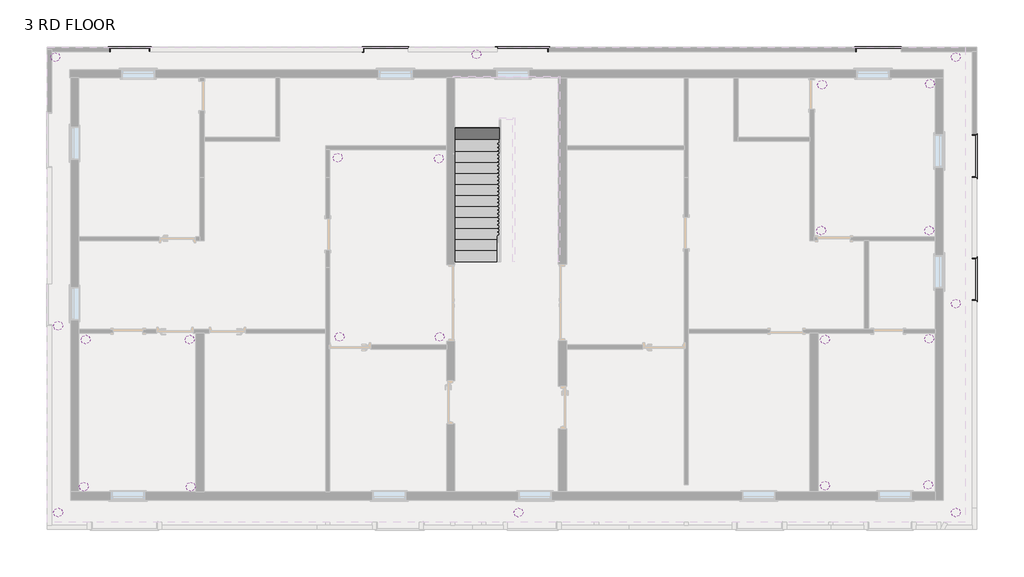
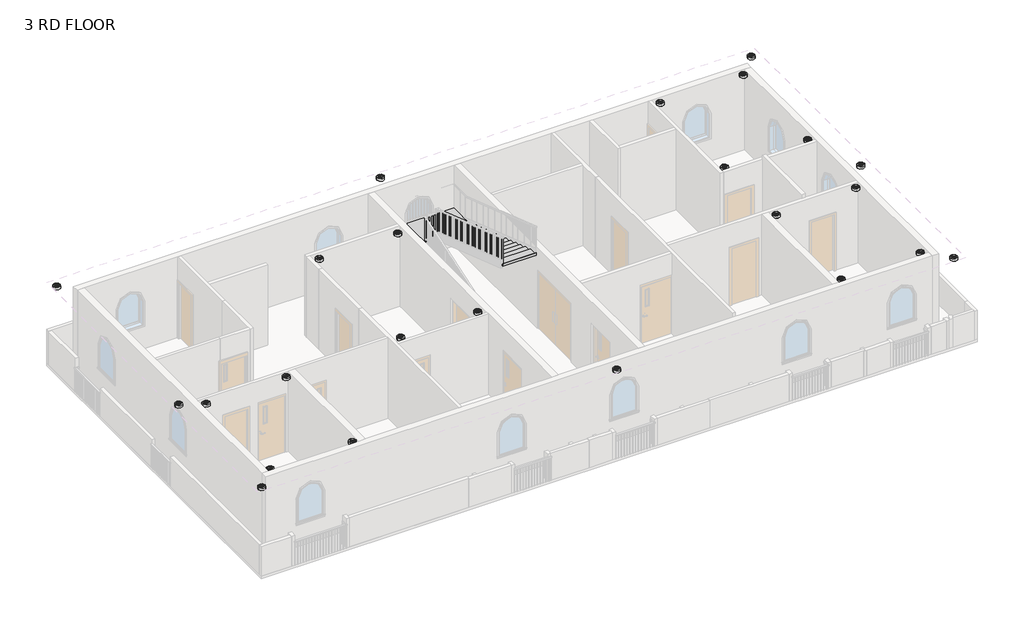
# One storey, part 6 of 7: 24 light fixtures, 6 railings, 1 stair flight.
"""IFC4 building model written with IfcOpenShell, lengths in millimetres."""

from ifc_helpers import new_model, si_unit, frame, origin, place, context, project, spatial, polyline, outline, extrude, faceted_brep, transform, mapped, element, save
from components import ceiling_light_flat_round_60w_120v_7c4c2a52, stair_flight_f733c31e

model = new_model("IFC4")

# Units and contexts
model_context = context("Model", 3, world=origin())
ifc_project = project(units=[si_unit("LENGTHUNIT", "METRE", prefix="MILLI")], contexts=[model_context])

# Site, building, storey
site = spatial("IfcSite", under=ifc_project)
building = spatial("IfcBuilding", under=site)
storey = spatial("IfcBuildingStorey", under=building, Name="3 RD FLOOR", Elevation=9601.2)

# Light fixtures
placement = place(None, origin())
ceiling_light_flat_round_60w_120v_shape = ceiling_light_flat_round_60w_120v_7c4c2a52(model_context)
element("IfcLightFixture", 1, ObjectType="Ceiling Light - Flat Round : 60W - 120V", at=placement, inside=storey, context=model_context, shape_type="MappedRepresentation", body=[
    mapped(ceiling_light_flat_round_60w_120v_shape, transform((-12872.3987925, 8203.3067329, 10210.8), x_axis=(1.0, 0.0, 0.0), y_axis=(0.0, 1.0, 0.0), z_axis=(0.0, 0.0, 1.0))),
])
element("IfcLightFixture", 2, ObjectType="Ceiling Light - Flat Round : 60W - 120V", at=placement, inside=storey, context=model_context, shape_type="MappedRepresentation", body=[
    mapped(ceiling_light_flat_round_60w_120v_shape, transform((-1251.8987998, 8279.5067329, 10210.8), x_axis=(1.0, 0.0, 0.0), y_axis=(0.0, 1.0, 0.0), z_axis=(0.0, 0.0, 1.0))),
])
element("IfcLightFixture", 3, ObjectType="Ceiling Light - Flat Round : 60W - 120V", at=placement, inside=storey, context=model_context, shape_type="MappedRepresentation", body=[
    mapped(ceiling_light_flat_round_60w_120v_shape, transform((11968.8012075, 8203.3067329, 10210.8), x_axis=(1.0, 0.0, 0.0), y_axis=(0.0, 1.0, 0.0), z_axis=(0.0, 0.0, 1.0))),
])
element("IfcLightFixture", 4, ObjectType="Ceiling Light - Flat Round : 60W - 120V", at=placement, inside=storey, context=model_context, shape_type="MappedRepresentation", body=[
    mapped(ceiling_light_flat_round_60w_120v_shape, transform((-12796.1987925, -4356.9932193, 10210.8), x_axis=(1.0, 0.0, 0.0), y_axis=(0.0, 1.0, 0.0), z_axis=(0.0, 0.0, 1.0))),
])
element("IfcLightFixture", 5, ObjectType="Ceiling Light - Flat Round : 60W - 120V", at=placement, inside=storey, context=model_context, shape_type="MappedRepresentation", body=[
    mapped(ceiling_light_flat_round_60w_120v_shape, transform((-96.7067989, -4356.9932193, 10210.8), x_axis=(1.0, 0.0, 0.0), y_axis=(0.0, 1.0, 0.0), z_axis=(0.0, 0.0, 1.0))),
])
element("IfcLightFixture", 6, ObjectType="Ceiling Light - Flat Round : 60W - 120V", at=placement, inside=storey, context=model_context, shape_type="MappedRepresentation", body=[
    mapped(ceiling_light_flat_round_60w_120v_shape, transform((11968.8012075, -4356.9932193, 10210.8), x_axis=(1.0, 0.0, 0.0), y_axis=(0.0, 1.0, 0.0), z_axis=(0.0, 0.0, 1.0))),
])
element("IfcLightFixture", 7, ObjectType="Ceiling Light - Flat Round : 60W - 120V", at=placement, inside=storey, context=model_context, shape_type="MappedRepresentation", body=[
    mapped(ceiling_light_flat_round_60w_120v_shape, transform((11968.8012075, 1402.4567334, 10210.8), x_axis=(1.0, 0.0, 0.0), y_axis=(0.0, 1.0, 0.0), z_axis=(0.0, 0.0, 1.0))),
])
element("IfcLightFixture", 8, ObjectType="Ceiling Light - Flat Round : 60W - 120V", at=placement, inside=storey, context=model_context, shape_type="MappedRepresentation", body=[
    mapped(ceiling_light_flat_round_60w_120v_shape, transform((-12796.1987925, 792.8567334, 10210.8), x_axis=(1.0, 0.0, 0.0), y_axis=(0.0, 1.0, 0.0), z_axis=(0.0, 0.0, 1.0))),
])
element("IfcLightFixture", 9, ObjectType="Ceiling Light - Flat Round : 60W - 120V", at=placement, inside=storey, context=model_context, shape_type="MappedRepresentation", body=[
    mapped(ceiling_light_flat_round_60w_120v_shape, transform((8279.4512079, 7441.3067329, 10210.8), x_axis=(1.0, 0.0, 0.0), y_axis=(0.0, 1.0, 0.0), z_axis=(0.0, 0.0, 1.0))),
])
element("IfcLightFixture", 10, ObjectType="Ceiling Light - Flat Round : 60W - 120V", at=placement, inside=storey, context=model_context, shape_type="MappedRepresentation", body=[
    mapped(ceiling_light_flat_round_60w_120v_shape, transform((11257.6012075, 7466.7067329, 10210.8), x_axis=(1.0, 0.0, 0.0), y_axis=(0.0, 1.0, 0.0), z_axis=(0.0, 0.0, 1.0))),
])
element("IfcLightFixture", 11, ObjectType="Ceiling Light - Flat Round : 60W - 120V", at=placement, inside=storey, context=model_context, shape_type="MappedRepresentation", body=[
    mapped(ceiling_light_flat_round_60w_120v_shape, transform((8254.0512079, 3421.7567332, 10210.8), x_axis=(1.0, 0.0, 0.0), y_axis=(0.0, 1.0, 0.0), z_axis=(0.0, 0.0, 1.0))),
])
element("IfcLightFixture", 12, ObjectType="Ceiling Light - Flat Round : 60W - 120V", at=placement, inside=storey, context=model_context, shape_type="MappedRepresentation", body=[
    mapped(ceiling_light_flat_round_60w_120v_shape, transform((11232.2012075, 3421.7567332, 10210.8), x_axis=(1.0, 0.0, 0.0), y_axis=(0.0, 1.0, 0.0), z_axis=(0.0, 0.0, 1.0))),
])
element("IfcLightFixture", 13, ObjectType="Ceiling Light - Flat Round : 60W - 120V", at=placement, inside=storey, context=model_context, shape_type="MappedRepresentation", body=[
    mapped(ceiling_light_flat_round_60w_120v_shape, transform((8362.0012079, 411.8567334, 10210.8), x_axis=(1.0, 0.0, 0.0), y_axis=(0.0, 1.0, 0.0), z_axis=(0.0, 0.0, 1.0))),
])
element("IfcLightFixture", 14, ObjectType="Ceiling Light - Flat Round : 60W - 120V", at=placement, inside=storey, context=model_context, shape_type="MappedRepresentation", body=[
    mapped(ceiling_light_flat_round_60w_120v_shape, transform((11232.2012075, 437.2567334, 10210.8), x_axis=(1.0, 0.0, 0.0), y_axis=(0.0, 1.0, 0.0), z_axis=(0.0, 0.0, 1.0))),
])
element("IfcLightFixture", 15, ObjectType="Ceiling Light - Flat Round : 60W - 120V", at=placement, inside=storey, context=model_context, shape_type="MappedRepresentation", body=[
    mapped(ceiling_light_flat_round_60w_120v_shape, transform((8362.0012079, -3620.3932193, 10210.8), x_axis=(1.0, 0.0, 0.0), y_axis=(0.0, 1.0, 0.0), z_axis=(0.0, 0.0, 1.0))),
])
element("IfcLightFixture", 16, ObjectType="Ceiling Light - Flat Round : 60W - 120V", at=placement, inside=storey, context=model_context, shape_type="MappedRepresentation", body=[
    mapped(ceiling_light_flat_round_60w_120v_shape, transform((11206.8012075, -3594.9932193, 10210.8), x_axis=(1.0, 0.0, 0.0), y_axis=(0.0, 1.0, 0.0), z_axis=(0.0, 0.0, 1.0))),
])
element("IfcLightFixture", 17, ObjectType="Ceiling Light - Flat Round : 60W - 120V", at=placement, inside=storey, context=model_context, shape_type="MappedRepresentation", body=[
    mapped(ceiling_light_flat_round_60w_120v_shape, transform((-12034.1987925, 411.8567334, 10210.8), x_axis=(1.0, 0.0, 0.0), y_axis=(0.0, 1.0, 0.0), z_axis=(0.0, 0.0, 1.0))),
])
element("IfcLightFixture", 18, ObjectType="Ceiling Light - Flat Round : 60W - 120V", at=placement, inside=storey, context=model_context, shape_type="MappedRepresentation", body=[
    mapped(ceiling_light_flat_round_60w_120v_shape, transform((-9163.9987992, 411.8567334, 10210.8), x_axis=(1.0, 0.0, 0.0), y_axis=(0.0, 1.0, 0.0), z_axis=(0.0, 0.0, 1.0))),
])
element("IfcLightFixture", 19, ObjectType="Ceiling Light - Flat Round : 60W - 120V", at=placement, inside=storey, context=model_context, shape_type="MappedRepresentation", body=[
    mapped(ceiling_light_flat_round_60w_120v_shape, transform((-12084.9987925, -3645.7932193, 10210.8), x_axis=(1.0, 0.0, 0.0), y_axis=(0.0, 1.0, 0.0), z_axis=(0.0, 0.0, 1.0))),
])
element("IfcLightFixture", 20, ObjectType="Ceiling Light - Flat Round : 60W - 120V", at=placement, inside=storey, context=model_context, shape_type="MappedRepresentation", body=[
    mapped(ceiling_light_flat_round_60w_120v_shape, transform((-9138.5987992, -3645.7932193, 10210.8), x_axis=(1.0, 0.0, 0.0), y_axis=(0.0, 1.0, 0.0), z_axis=(0.0, 0.0, 1.0))),
])
element("IfcLightFixture", 21, ObjectType="Ceiling Light - Flat Round : 60W - 120V", at=placement, inside=storey, context=model_context, shape_type="MappedRepresentation", body=[
    mapped(ceiling_light_flat_round_60w_120v_shape, transform((-5080.9487995, 5428.3567329, 10210.8), x_axis=(1.0, 0.0, 0.0), y_axis=(0.0, 1.0, 0.0), z_axis=(0.0, 0.0, 1.0))),
])
element("IfcLightFixture", 22, ObjectType="Ceiling Light - Flat Round : 60W - 120V", at=placement, inside=storey, context=model_context, shape_type="MappedRepresentation", body=[
    mapped(ceiling_light_flat_round_60w_120v_shape, transform((-2293.2987998, 5402.9567329, 10210.8), x_axis=(1.0, 0.0, 0.0), y_axis=(0.0, 1.0, 0.0), z_axis=(0.0, 0.0, 1.0))),
])
element("IfcLightFixture", 23, ObjectType="Ceiling Light - Flat Round : 60W - 120V", at=placement, inside=storey, context=model_context, shape_type="MappedRepresentation", body=[
    mapped(ceiling_light_flat_round_60w_120v_shape, transform((-5030.1487995, 488.0567334, 10210.8), x_axis=(1.0, 0.0, 0.0), y_axis=(0.0, 1.0, 0.0), z_axis=(0.0, 0.0, 1.0))),
])
element("IfcLightFixture", 24, ObjectType="Ceiling Light - Flat Round : 60W - 120V", at=placement, inside=storey, context=model_context, shape_type="MappedRepresentation", body=[
    mapped(ceiling_light_flat_round_60w_120v_shape, transform((-2267.8987998, 488.0567334, 10210.8), x_axis=(1.0, 0.0, 0.0), y_axis=(0.0, 1.0, 0.0), z_axis=(0.0, 0.0, 1.0))),
])

# Railings
element("IfcRailing", 25, ObjectType="Handrail - Rectangular", at=placement, inside=storey, context=model_context, shape_type="SolidModel", body=[
    faceted_brep([(-11412.4067989, 8355.7067329, 10515.6), (-11412.4067989, 8355.7067329, 10464.8), (-11361.6067989, 8355.7067329, 10464.8), (-11361.6067989, 8355.7067329, 10515.6), (-11412.4067989, 8495.4067329, 10515.6), (-11412.4067989, 8495.4067329, 10464.8), (-11361.6067989, 8444.6067329, 10464.8), (-11361.6067989, 8444.6067329, 10515.6), (-10231.3067989, 8495.4067329, 10515.6), (-10231.3067989, 8495.4067329, 10464.8), (-10282.1067989, 8444.6067329, 10464.8), (-10282.1067989, 8444.6067329, 10515.6), (-10231.3067989, 8368.4067329, 10515.6), (-10282.1067989, 8368.4067329, 10515.6), (-10282.1067989, 8368.4067329, 10464.8), (-10231.3067989, 8368.4067329, 10464.8)], [[[0, 1, 2, 3]], [[1, 0, 4, 5]], [[2, 1, 5, 6]], [[3, 2, 6, 7]], [[0, 3, 7, 4]], [[5, 4, 8, 9]], [[6, 5, 9, 10]], [[7, 6, 10, 11]], [[4, 7, 11, 8]], [[12, 13, 14, 15]], [[9, 8, 12, 15]], [[10, 9, 15, 14]], [[11, 10, 14, 13]], [[8, 11, 13, 12]]]),
    extrude(outline(polyline([(-10278.9317989, 8460.4817329), (-10278.9317989, 8479.5317329), (-10259.8817989, 8479.5317329), (-10259.8817989, 8460.4817329), (-10278.9317989, 8460.4817329)])), frame((0.0, 0.0, 9601.2), z_axis=(0.0, 0.0, 1.0), x_axis=(1.0, 0.0, 0.0)), (0.0, 0.0, 1.0), 863.6),
    extrude(outline(polyline([(-10380.5317989, 8460.4817329), (-10380.5317989, 8479.5317329), (-10361.4817989, 8479.5317329), (-10361.4817989, 8460.4817329), (-10380.5317989, 8460.4817329)])), frame((0.0, 0.0, 9601.2), z_axis=(0.0, 0.0, 1.0), x_axis=(1.0, 0.0, 0.0)), (0.0, 0.0, 1.0), 863.6),
    extrude(outline(polyline([(-10482.1317989, 8460.4817329), (-10482.1317989, 8479.5317329), (-10463.0817989, 8479.5317329), (-10463.0817989, 8460.4817329), (-10482.1317989, 8460.4817329)])), frame((0.0, 0.0, 9601.2), z_axis=(0.0, 0.0, 1.0), x_axis=(1.0, 0.0, 0.0)), (0.0, 0.0, 1.0), 863.6),
    extrude(outline(polyline([(-10583.7317989, 8460.4817329), (-10583.7317989, 8479.5317329), (-10564.6817989, 8479.5317329), (-10564.6817989, 8460.4817329), (-10583.7317989, 8460.4817329)])), frame((0.0, 0.0, 9601.2), z_axis=(0.0, 0.0, 1.0), x_axis=(1.0, 0.0, 0.0)), (0.0, 0.0, 1.0), 863.6),
    extrude(outline(polyline([(-10685.3317989, 8460.4817329), (-10685.3317989, 8479.5317329), (-10666.2817989, 8479.5317329), (-10666.2817989, 8460.4817329), (-10685.3317989, 8460.4817329)])), frame((0.0, 0.0, 9601.2), z_axis=(0.0, 0.0, 1.0), x_axis=(1.0, 0.0, 0.0)), (0.0, 0.0, 1.0), 863.6),
    extrude(outline(polyline([(-10786.9317989, 8460.4817329), (-10786.9317989, 8479.5317329), (-10767.8817989, 8479.5317329), (-10767.8817989, 8460.4817329), (-10786.9317989, 8460.4817329)])), frame((0.0, 0.0, 9601.2), z_axis=(0.0, 0.0, 1.0), x_axis=(1.0, 0.0, 0.0)), (0.0, 0.0, 1.0), 863.6),
    extrude(outline(polyline([(-10888.5317989, 8460.4817329), (-10888.5317989, 8479.5317329), (-10869.4817989, 8479.5317329), (-10869.4817989, 8460.4817329), (-10888.5317989, 8460.4817329)])), frame((0.0, 0.0, 9601.2), z_axis=(0.0, 0.0, 1.0), x_axis=(1.0, 0.0, 0.0)), (0.0, 0.0, 1.0), 863.6),
    extrude(outline(polyline([(-10990.1317989, 8460.4817329), (-10990.1317989, 8479.5317329), (-10971.0817989, 8479.5317329), (-10971.0817989, 8460.4817329), (-10990.1317989, 8460.4817329)])), frame((0.0, 0.0, 9601.2), z_axis=(0.0, 0.0, 1.0), x_axis=(1.0, 0.0, 0.0)), (0.0, 0.0, 1.0), 863.6),
    extrude(outline(polyline([(-11091.7317989, 8460.4817329), (-11091.7317989, 8479.5317329), (-11072.6817989, 8479.5317329), (-11072.6817989, 8460.4817329), (-11091.7317989, 8460.4817329)])), frame((0.0, 0.0, 9601.2), z_axis=(0.0, 0.0, 1.0), x_axis=(1.0, 0.0, 0.0)), (0.0, 0.0, 1.0), 863.6),
    extrude(outline(polyline([(-11193.3317989, 8460.4817329), (-11193.3317989, 8479.5317329), (-11174.2817989, 8479.5317329), (-11174.2817989, 8460.4817329), (-11193.3317989, 8460.4817329)])), frame((0.0, 0.0, 9601.2), z_axis=(0.0, 0.0, 1.0), x_axis=(1.0, 0.0, 0.0)), (0.0, 0.0, 1.0), 863.6),
    extrude(outline(polyline([(-11294.9317989, 8460.4817329), (-11294.9317989, 8479.5317329), (-11275.8817989, 8479.5317329), (-11275.8817989, 8460.4817329), (-11294.9317989, 8460.4817329)])), frame((0.0, 0.0, 9601.2), z_axis=(0.0, 0.0, 1.0), x_axis=(1.0, 0.0, 0.0)), (0.0, 0.0, 1.0), 863.6),
    extrude(outline(polyline([(-11377.4817989, 8447.7817329), (-11396.5317989, 8447.7817329), (-11396.5317989, 8466.8317329), (-11377.4817989, 8466.8317329), (-11377.4817989, 8447.7817329)])), frame((0.0, 0.0, 9601.2), z_axis=(0.0, 0.0, 1.0), x_axis=(1.0, 0.0, 0.0)), (0.0, 0.0, 1.0), 863.6),
    extrude(outline(polyline([(-10266.2317989, 8460.4817329), (-10266.2317989, 8479.5317329), (-10247.1817989, 8479.5317329), (-10247.1817989, 8460.4817329), (-10266.2317989, 8460.4817329)])), frame((0.0, 0.0, 9601.2), z_axis=(0.0, 0.0, 1.0), x_axis=(1.0, 0.0, 0.0)), (0.0, 0.0, 1.0), 863.6),
    extrude(outline(polyline([(-11377.4817989, 8460.4817329), (-11396.5317989, 8460.4817329), (-11396.5317989, 8479.5317329), (-11377.4817989, 8479.5317329), (-11377.4817989, 8460.4817329)])), frame((0.0, 0.0, 9601.2), z_axis=(0.0, 0.0, 1.0), x_axis=(1.0, 0.0, 0.0)), (0.0, 0.0, 1.0), 863.6),
    extrude(outline(polyline([(-10266.2317989, 8387.4567329), (-10247.1817989, 8387.4567329), (-10247.1817989, 8368.4067329), (-10266.2317989, 8368.4067329), (-10266.2317989, 8387.4567329)])), frame((0.0, 0.0, 9601.2), z_axis=(0.0, 0.0, 1.0), x_axis=(1.0, 0.0, 0.0)), (0.0, 0.0, 1.0), 863.6),
    extrude(outline(polyline([(-11377.4817989, 8355.7067329), (-11396.5317989, 8355.7067329), (-11396.5317989, 8374.7567329), (-11377.4817989, 8374.7567329), (-11377.4817989, 8355.7067329)])), frame((0.0, 0.0, 9601.2), z_axis=(0.0, 0.0, 1.0), x_axis=(1.0, 0.0, 0.0)), (0.0, 0.0, 1.0), 863.6),
])
element("IfcRailing", 26, ObjectType="Handrail - Rectangular", at=placement, inside=storey, context=model_context, shape_type="SolidModel", body=[
    faceted_brep([(-4407.8487992, 8336.6567329, 10515.6), (-4407.8487992, 8336.6567329, 10464.8), (-4357.0487992, 8336.6567329, 10464.8), (-4357.0487992, 8336.6567329, 10515.6), (-4407.8487992, 8495.4067329, 10515.6), (-4407.8487992, 8495.4067329, 10464.8), (-4357.0487992, 8444.6067329, 10464.8), (-4357.0487992, 8444.6067329, 10515.6), (-3120.4490672, 8495.4067329, 10515.6), (-3120.4490672, 8444.6067329, 10515.6), (-3120.4490672, 8444.6067329, 10464.8), (-3120.4490672, 8495.4067329, 10464.8)], [[[0, 1, 2, 3]], [[1, 0, 4, 5]], [[2, 1, 5, 6]], [[3, 2, 6, 7]], [[0, 3, 7, 4]], [[8, 9, 10, 11]], [[5, 4, 8, 11]], [[6, 5, 11, 10]], [[7, 6, 10, 9]], [[4, 7, 9, 8]]]),
    extrude(outline(polyline([(-3172.7737992, 8460.4817329), (-3172.7737992, 8479.5317329), (-3153.7237992, 8479.5317329), (-3153.7237992, 8460.4817329), (-3172.7737992, 8460.4817329)])), frame((0.0, 0.0, 9601.2), z_axis=(0.0, 0.0, 1.0), x_axis=(1.0, 0.0, 0.0)), (0.0, 0.0, 1.0), 863.6),
    extrude(outline(polyline([(-3274.3737992, 8460.4817329), (-3274.3737992, 8479.5317329), (-3255.3237992, 8479.5317329), (-3255.3237992, 8460.4817329), (-3274.3737992, 8460.4817329)])), frame((0.0, 0.0, 9601.2), z_axis=(0.0, 0.0, 1.0), x_axis=(1.0, 0.0, 0.0)), (0.0, 0.0, 1.0), 863.6),
    extrude(outline(polyline([(-3375.9737992, 8460.4817329), (-3375.9737992, 8479.5317329), (-3356.9237992, 8479.5317329), (-3356.9237992, 8460.4817329), (-3375.9737992, 8460.4817329)])), frame((0.0, 0.0, 9601.2), z_axis=(0.0, 0.0, 1.0), x_axis=(1.0, 0.0, 0.0)), (0.0, 0.0, 1.0), 863.6),
    extrude(outline(polyline([(-3477.5737992, 8460.4817329), (-3477.5737992, 8479.5317329), (-3458.5237992, 8479.5317329), (-3458.5237992, 8460.4817329), (-3477.5737992, 8460.4817329)])), frame((0.0, 0.0, 9601.2), z_axis=(0.0, 0.0, 1.0), x_axis=(1.0, 0.0, 0.0)), (0.0, 0.0, 1.0), 863.6),
    extrude(outline(polyline([(-3579.1737992, 8460.4817329), (-3579.1737992, 8479.5317329), (-3560.1237992, 8479.5317329), (-3560.1237992, 8460.4817329), (-3579.1737992, 8460.4817329)])), frame((0.0, 0.0, 9601.2), z_axis=(0.0, 0.0, 1.0), x_axis=(1.0, 0.0, 0.0)), (0.0, 0.0, 1.0), 863.6),
    extrude(outline(polyline([(-3680.7737992, 8460.4817329), (-3680.7737992, 8479.5317329), (-3661.7237992, 8479.5317329), (-3661.7237992, 8460.4817329), (-3680.7737992, 8460.4817329)])), frame((0.0, 0.0, 9601.2), z_axis=(0.0, 0.0, 1.0), x_axis=(1.0, 0.0, 0.0)), (0.0, 0.0, 1.0), 863.6),
    extrude(outline(polyline([(-3782.3737992, 8460.4817329), (-3782.3737992, 8479.5317329), (-3763.3237992, 8479.5317329), (-3763.3237992, 8460.4817329), (-3782.3737992, 8460.4817329)])), frame((0.0, 0.0, 9601.2), z_axis=(0.0, 0.0, 1.0), x_axis=(1.0, 0.0, 0.0)), (0.0, 0.0, 1.0), 863.6),
    extrude(outline(polyline([(-3883.9737992, 8460.4817329), (-3883.9737992, 8479.5317329), (-3864.9237992, 8479.5317329), (-3864.9237992, 8460.4817329), (-3883.9737992, 8460.4817329)])), frame((0.0, 0.0, 9601.2), z_axis=(0.0, 0.0, 1.0), x_axis=(1.0, 0.0, 0.0)), (0.0, 0.0, 1.0), 863.6),
    extrude(outline(polyline([(-3985.5737992, 8460.4817329), (-3985.5737992, 8479.5317329), (-3966.5237992, 8479.5317329), (-3966.5237992, 8460.4817329), (-3985.5737992, 8460.4817329)])), frame((0.0, 0.0, 9601.2), z_axis=(0.0, 0.0, 1.0), x_axis=(1.0, 0.0, 0.0)), (0.0, 0.0, 1.0), 863.6),
    extrude(outline(polyline([(-4087.1737992, 8460.4817329), (-4087.1737992, 8479.5317329), (-4068.1237992, 8479.5317329), (-4068.1237992, 8460.4817329), (-4087.1737992, 8460.4817329)])), frame((0.0, 0.0, 9601.2), z_axis=(0.0, 0.0, 1.0), x_axis=(1.0, 0.0, 0.0)), (0.0, 0.0, 1.0), 863.6),
    extrude(outline(polyline([(-4188.7737992, 8460.4817329), (-4188.7737992, 8479.5317329), (-4169.7237992, 8479.5317329), (-4169.7237992, 8460.4817329), (-4188.7737992, 8460.4817329)])), frame((0.0, 0.0, 9601.2), z_axis=(0.0, 0.0, 1.0), x_axis=(1.0, 0.0, 0.0)), (0.0, 0.0, 1.0), 863.6),
    extrude(outline(polyline([(-4290.3737992, 8460.4817329), (-4290.3737992, 8479.5317329), (-4271.3237992, 8479.5317329), (-4271.3237992, 8460.4817329), (-4290.3737992, 8460.4817329)])), frame((0.0, 0.0, 9601.2), z_axis=(0.0, 0.0, 1.0), x_axis=(1.0, 0.0, 0.0)), (0.0, 0.0, 1.0), 863.6),
    extrude(outline(polyline([(-4372.9237992, 8428.7317329), (-4391.9737992, 8428.7317329), (-4391.9737992, 8447.7817329), (-4372.9237992, 8447.7817329), (-4372.9237992, 8428.7317329)])), frame((0.0, 0.0, 9601.2), z_axis=(0.0, 0.0, 1.0), x_axis=(1.0, 0.0, 0.0)), (0.0, 0.0, 1.0), 863.6),
    extrude(outline(polyline([(-4372.9237992, 8460.4817329), (-4391.9737992, 8460.4817329), (-4391.9737992, 8479.5317329), (-4372.9237992, 8479.5317329), (-4372.9237992, 8460.4817329)])), frame((0.0, 0.0, 9601.2), z_axis=(0.0, 0.0, 1.0), x_axis=(1.0, 0.0, 0.0)), (0.0, 0.0, 1.0), 863.6),
    extrude(outline(polyline([(-3139.4990672, 8460.4817329), (-3139.4990672, 8479.5317329), (-3120.4490672, 8479.5317329), (-3120.4490672, 8460.4817329), (-3139.4990672, 8460.4817329)])), frame((0.0, 0.0, 9601.2), z_axis=(0.0, 0.0, 1.0), x_axis=(1.0, 0.0, 0.0)), (0.0, 0.0, 1.0), 863.6),
    extrude(outline(polyline([(-4372.9237992, 8336.6567329), (-4391.9737992, 8336.6567329), (-4391.9737992, 8355.7067329), (-4372.9237992, 8355.7067329), (-4372.9237992, 8336.6567329)])), frame((0.0, 0.0, 9601.2), z_axis=(0.0, 0.0, 1.0), x_axis=(1.0, 0.0, 0.0)), (0.0, 0.0, 1.0), 863.6),
])
element("IfcRailing", 27, ObjectType="Handrail - Rectangular", at=placement, inside=storey, context=model_context, shape_type="SolidModel", body=[
    faceted_brep([(-732.8490672, 8355.7067329, 10515.6), (-732.8490672, 8355.7067329, 10464.8), (-682.0490672, 8355.7067329, 10464.8), (-682.0490672, 8355.7067329, 10515.6), (-732.8490672, 8495.4067329, 10515.6), (-732.8490672, 8495.4067329, 10464.8), (-682.0490672, 8444.6067329, 10464.8), (-682.0490672, 8444.6067329, 10515.6), (766.8932011, 8495.4067329, 10515.6), (766.8932011, 8495.4067329, 10464.8), (716.0932011, 8444.6067329, 10464.8), (716.0932011, 8444.6067329, 10515.6), (766.8932011, 8355.7067329, 10515.6), (716.0932011, 8355.7067329, 10515.6), (716.0932011, 8355.7067329, 10464.8), (766.8932011, 8355.7067329, 10464.8)], [[[0, 1, 2, 3]], [[1, 0, 4, 5]], [[2, 1, 5, 6]], [[3, 2, 6, 7]], [[0, 3, 7, 4]], [[5, 4, 8, 9]], [[6, 5, 9, 10]], [[7, 6, 10, 11]], [[4, 7, 11, 8]], [[12, 13, 14, 15]], [[9, 8, 12, 15]], [[10, 9, 15, 14]], [[11, 10, 14, 13]], [[8, 11, 13, 12]]]),
    extrude(outline(polyline([(731.9682011, 8377.9317329), (751.0182011, 8377.9317329), (751.0182011, 8358.8817329), (731.9682011, 8358.8817329), (731.9682011, 8377.9317329)])), frame((0.0, 0.0, 9601.2), z_axis=(0.0, 0.0, 1.0), x_axis=(1.0, 0.0, 0.0)), (0.0, 0.0, 1.0), 863.6),
    extrude(outline(polyline([(705.4259328, 8460.4817329), (705.4259328, 8479.5317329), (724.4759328, 8479.5317329), (724.4759328, 8460.4817329), (705.4259328, 8460.4817329)])), frame((0.0, 0.0, 9601.2), z_axis=(0.0, 0.0, 1.0), x_axis=(1.0, 0.0, 0.0)), (0.0, 0.0, 1.0), 863.6),
    extrude(outline(polyline([(603.8259328, 8460.4817329), (603.8259328, 8479.5317329), (622.8759328, 8479.5317329), (622.8759328, 8460.4817329), (603.8259328, 8460.4817329)])), frame((0.0, 0.0, 9601.2), z_axis=(0.0, 0.0, 1.0), x_axis=(1.0, 0.0, 0.0)), (0.0, 0.0, 1.0), 863.6),
    extrude(outline(polyline([(502.2259328, 8460.4817329), (502.2259328, 8479.5317329), (521.2759328, 8479.5317329), (521.2759328, 8460.4817329), (502.2259328, 8460.4817329)])), frame((0.0, 0.0, 9601.2), z_axis=(0.0, 0.0, 1.0), x_axis=(1.0, 0.0, 0.0)), (0.0, 0.0, 1.0), 863.6),
    extrude(outline(polyline([(400.6259328, 8460.4817329), (400.6259328, 8479.5317329), (419.6759328, 8479.5317329), (419.6759328, 8460.4817329), (400.6259328, 8460.4817329)])), frame((0.0, 0.0, 9601.2), z_axis=(0.0, 0.0, 1.0), x_axis=(1.0, 0.0, 0.0)), (0.0, 0.0, 1.0), 863.6),
    extrude(outline(polyline([(299.0259328, 8460.4817329), (299.0259328, 8479.5317329), (318.0759328, 8479.5317329), (318.0759328, 8460.4817329), (299.0259328, 8460.4817329)])), frame((0.0, 0.0, 9601.2), z_axis=(0.0, 0.0, 1.0), x_axis=(1.0, 0.0, 0.0)), (0.0, 0.0, 1.0), 863.6),
    extrude(outline(polyline([(197.4259328, 8460.4817329), (197.4259328, 8479.5317329), (216.4759328, 8479.5317329), (216.4759328, 8460.4817329), (197.4259328, 8460.4817329)])), frame((0.0, 0.0, 9601.2), z_axis=(0.0, 0.0, 1.0), x_axis=(1.0, 0.0, 0.0)), (0.0, 0.0, 1.0), 863.6),
    extrude(outline(polyline([(95.8259328, 8460.4817329), (95.8259328, 8479.5317329), (114.8759328, 8479.5317329), (114.8759328, 8460.4817329), (95.8259328, 8460.4817329)])), frame((0.0, 0.0, 9601.2), z_axis=(0.0, 0.0, 1.0), x_axis=(1.0, 0.0, 0.0)), (0.0, 0.0, 1.0), 863.6),
    extrude(outline(polyline([(-5.7740672, 8460.4817329), (-5.7740672, 8479.5317329), (13.2759328, 8479.5317329), (13.2759328, 8460.4817329), (-5.7740672, 8460.4817329)])), frame((0.0, 0.0, 9601.2), z_axis=(0.0, 0.0, 1.0), x_axis=(1.0, 0.0, 0.0)), (0.0, 0.0, 1.0), 863.6),
    extrude(outline(polyline([(-107.3740672, 8460.4817329), (-107.3740672, 8479.5317329), (-88.3240672, 8479.5317329), (-88.3240672, 8460.4817329), (-107.3740672, 8460.4817329)])), frame((0.0, 0.0, 9601.2), z_axis=(0.0, 0.0, 1.0), x_axis=(1.0, 0.0, 0.0)), (0.0, 0.0, 1.0), 863.6),
    extrude(outline(polyline([(-208.9740672, 8460.4817329), (-208.9740672, 8479.5317329), (-189.9240672, 8479.5317329), (-189.9240672, 8460.4817329), (-208.9740672, 8460.4817329)])), frame((0.0, 0.0, 9601.2), z_axis=(0.0, 0.0, 1.0), x_axis=(1.0, 0.0, 0.0)), (0.0, 0.0, 1.0), 863.6),
    extrude(outline(polyline([(-310.5740672, 8460.4817329), (-310.5740672, 8479.5317329), (-291.5240672, 8479.5317329), (-291.5240672, 8460.4817329), (-310.5740672, 8460.4817329)])), frame((0.0, 0.0, 9601.2), z_axis=(0.0, 0.0, 1.0), x_axis=(1.0, 0.0, 0.0)), (0.0, 0.0, 1.0), 863.6),
    extrude(outline(polyline([(-412.1740672, 8460.4817329), (-412.1740672, 8479.5317329), (-393.1240672, 8479.5317329), (-393.1240672, 8460.4817329), (-412.1740672, 8460.4817329)])), frame((0.0, 0.0, 9601.2), z_axis=(0.0, 0.0, 1.0), x_axis=(1.0, 0.0, 0.0)), (0.0, 0.0, 1.0), 863.6),
    extrude(outline(polyline([(-513.7740672, 8460.4817329), (-513.7740672, 8479.5317329), (-494.7240672, 8479.5317329), (-494.7240672, 8460.4817329), (-513.7740672, 8460.4817329)])), frame((0.0, 0.0, 9601.2), z_axis=(0.0, 0.0, 1.0), x_axis=(1.0, 0.0, 0.0)), (0.0, 0.0, 1.0), 863.6),
    extrude(outline(polyline([(-615.3740672, 8460.4817329), (-615.3740672, 8479.5317329), (-596.3240672, 8479.5317329), (-596.3240672, 8460.4817329), (-615.3740672, 8460.4817329)])), frame((0.0, 0.0, 9601.2), z_axis=(0.0, 0.0, 1.0), x_axis=(1.0, 0.0, 0.0)), (0.0, 0.0, 1.0), 863.6),
    extrude(outline(polyline([(-697.9240672, 8447.7817329), (-716.9740672, 8447.7817329), (-716.9740672, 8466.8317329), (-697.9240672, 8466.8317329), (-697.9240672, 8447.7817329)])), frame((0.0, 0.0, 9601.2), z_axis=(0.0, 0.0, 1.0), x_axis=(1.0, 0.0, 0.0)), (0.0, 0.0, 1.0), 863.6),
    extrude(outline(polyline([(731.9682011, 8460.4817329), (731.9682011, 8479.5317329), (751.0182011, 8479.5317329), (751.0182011, 8460.4817329), (731.9682011, 8460.4817329)])), frame((0.0, 0.0, 9601.2), z_axis=(0.0, 0.0, 1.0), x_axis=(1.0, 0.0, 0.0)), (0.0, 0.0, 1.0), 863.6),
    extrude(outline(polyline([(-697.9240672, 8460.4817329), (-716.9740672, 8460.4817329), (-716.9740672, 8479.5317329), (-697.9240672, 8479.5317329), (-697.9240672, 8460.4817329)])), frame((0.0, 0.0, 9601.2), z_axis=(0.0, 0.0, 1.0), x_axis=(1.0, 0.0, 0.0)), (0.0, 0.0, 1.0), 863.6),
    extrude(outline(polyline([(731.9682011, 8374.7567329), (751.0182011, 8374.7567329), (751.0182011, 8355.7067329), (731.9682011, 8355.7067329), (731.9682011, 8374.7567329)])), frame((0.0, 0.0, 9601.2), z_axis=(0.0, 0.0, 1.0), x_axis=(1.0, 0.0, 0.0)), (0.0, 0.0, 1.0), 863.6),
    extrude(outline(polyline([(-697.9240672, 8355.7067329), (-716.9740672, 8355.7067329), (-716.9740672, 8374.7567329), (-697.9240672, 8374.7567329), (-697.9240672, 8355.7067329)])), frame((0.0, 0.0, 9601.2), z_axis=(0.0, 0.0, 1.0), x_axis=(1.0, 0.0, 0.0)), (0.0, 0.0, 1.0), 863.6),
])
element("IfcRailing", 28, ObjectType="Handrail - Rectangular", at=placement, inside=storey, context=model_context, shape_type="SolidModel", body=[
    faceted_brep([(9174.2932011, 8355.7067329, 10515.6), (9174.2932011, 8355.7067329, 10464.8), (9225.0932011, 8355.7067329, 10464.8), (9225.0932011, 8355.7067329, 10515.6), (9174.2932011, 8495.4067329, 10515.6), (9174.2932011, 8495.4067329, 10464.8), (9225.0932011, 8444.6067329, 10464.8), (9225.0932011, 8444.6067329, 10515.6), (10462.2009401, 8495.4067329, 10515.6), (10462.2009401, 8444.6067329, 10515.6), (10462.2009401, 8444.6067329, 10464.8), (10462.2009401, 8495.4067329, 10464.8)], [[[0, 1, 2, 3]], [[1, 0, 4, 5]], [[2, 1, 5, 6]], [[3, 2, 6, 7]], [[0, 3, 7, 4]], [[8, 9, 10, 11]], [[5, 4, 8, 11]], [[6, 5, 11, 10]], [[7, 6, 10, 9]], [[4, 7, 9, 8]]]),
    extrude(outline(polyline([(10409.3682011, 8460.4817329), (10409.3682011, 8479.5317329), (10428.4182011, 8479.5317329), (10428.4182011, 8460.4817329), (10409.3682011, 8460.4817329)])), frame((0.0, 0.0, 9601.2), z_axis=(0.0, 0.0, 1.0), x_axis=(1.0, 0.0, 0.0)), (0.0, 0.0, 1.0), 863.6),
    extrude(outline(polyline([(10307.7682011, 8460.4817329), (10307.7682011, 8479.5317329), (10326.8182011, 8479.5317329), (10326.8182011, 8460.4817329), (10307.7682011, 8460.4817329)])), frame((0.0, 0.0, 9601.2), z_axis=(0.0, 0.0, 1.0), x_axis=(1.0, 0.0, 0.0)), (0.0, 0.0, 1.0), 863.6),
    extrude(outline(polyline([(10206.1682011, 8460.4817329), (10206.1682011, 8479.5317329), (10225.2182011, 8479.5317329), (10225.2182011, 8460.4817329), (10206.1682011, 8460.4817329)])), frame((0.0, 0.0, 9601.2), z_axis=(0.0, 0.0, 1.0), x_axis=(1.0, 0.0, 0.0)), (0.0, 0.0, 1.0), 863.6),
    extrude(outline(polyline([(10104.5682011, 8460.4817329), (10104.5682011, 8479.5317329), (10123.6182011, 8479.5317329), (10123.6182011, 8460.4817329), (10104.5682011, 8460.4817329)])), frame((0.0, 0.0, 9601.2), z_axis=(0.0, 0.0, 1.0), x_axis=(1.0, 0.0, 0.0)), (0.0, 0.0, 1.0), 863.6),
    extrude(outline(polyline([(10002.9682011, 8460.4817329), (10002.9682011, 8479.5317329), (10022.0182011, 8479.5317329), (10022.0182011, 8460.4817329), (10002.9682011, 8460.4817329)])), frame((0.0, 0.0, 9601.2), z_axis=(0.0, 0.0, 1.0), x_axis=(1.0, 0.0, 0.0)), (0.0, 0.0, 1.0), 863.6),
    extrude(outline(polyline([(9901.3682011, 8460.4817329), (9901.3682011, 8479.5317329), (9920.4182011, 8479.5317329), (9920.4182011, 8460.4817329), (9901.3682011, 8460.4817329)])), frame((0.0, 0.0, 9601.2), z_axis=(0.0, 0.0, 1.0), x_axis=(1.0, 0.0, 0.0)), (0.0, 0.0, 1.0), 863.6),
    extrude(outline(polyline([(9799.7682011, 8460.4817329), (9799.7682011, 8479.5317329), (9818.8182011, 8479.5317329), (9818.8182011, 8460.4817329), (9799.7682011, 8460.4817329)])), frame((0.0, 0.0, 9601.2), z_axis=(0.0, 0.0, 1.0), x_axis=(1.0, 0.0, 0.0)), (0.0, 0.0, 1.0), 863.6),
    extrude(outline(polyline([(9698.1682011, 8460.4817329), (9698.1682011, 8479.5317329), (9717.2182011, 8479.5317329), (9717.2182011, 8460.4817329), (9698.1682011, 8460.4817329)])), frame((0.0, 0.0, 9601.2), z_axis=(0.0, 0.0, 1.0), x_axis=(1.0, 0.0, 0.0)), (0.0, 0.0, 1.0), 863.6),
    extrude(outline(polyline([(9596.5682011, 8460.4817329), (9596.5682011, 8479.5317329), (9615.6182011, 8479.5317329), (9615.6182011, 8460.4817329), (9596.5682011, 8460.4817329)])), frame((0.0, 0.0, 9601.2), z_axis=(0.0, 0.0, 1.0), x_axis=(1.0, 0.0, 0.0)), (0.0, 0.0, 1.0), 863.6),
    extrude(outline(polyline([(9494.9682011, 8460.4817329), (9494.9682011, 8479.5317329), (9514.0182011, 8479.5317329), (9514.0182011, 8460.4817329), (9494.9682011, 8460.4817329)])), frame((0.0, 0.0, 9601.2), z_axis=(0.0, 0.0, 1.0), x_axis=(1.0, 0.0, 0.0)), (0.0, 0.0, 1.0), 863.6),
    extrude(outline(polyline([(9393.3682011, 8460.4817329), (9393.3682011, 8479.5317329), (9412.4182011, 8479.5317329), (9412.4182011, 8460.4817329), (9393.3682011, 8460.4817329)])), frame((0.0, 0.0, 9601.2), z_axis=(0.0, 0.0, 1.0), x_axis=(1.0, 0.0, 0.0)), (0.0, 0.0, 1.0), 863.6),
    extrude(outline(polyline([(9291.7682011, 8460.4817329), (9291.7682011, 8479.5317329), (9310.8182011, 8479.5317329), (9310.8182011, 8460.4817329), (9291.7682011, 8460.4817329)])), frame((0.0, 0.0, 9601.2), z_axis=(0.0, 0.0, 1.0), x_axis=(1.0, 0.0, 0.0)), (0.0, 0.0, 1.0), 863.6),
    extrude(outline(polyline([(9209.2182011, 8447.7817329), (9190.1682011, 8447.7817329), (9190.1682011, 8466.8317329), (9209.2182011, 8466.8317329), (9209.2182011, 8447.7817329)])), frame((0.0, 0.0, 9601.2), z_axis=(0.0, 0.0, 1.0), x_axis=(1.0, 0.0, 0.0)), (0.0, 0.0, 1.0), 863.6),
    extrude(outline(polyline([(9209.2182011, 8460.4817329), (9190.1682011, 8460.4817329), (9190.1682011, 8479.5317329), (9209.2182011, 8479.5317329), (9209.2182011, 8460.4817329)])), frame((0.0, 0.0, 9601.2), z_axis=(0.0, 0.0, 1.0), x_axis=(1.0, 0.0, 0.0)), (0.0, 0.0, 1.0), 863.6),
    extrude(outline(polyline([(10443.1509401, 8460.4817329), (10443.1509401, 8479.5317329), (10462.2009401, 8479.5317329), (10462.2009401, 8460.4817329), (10443.1509401, 8460.4817329)])), frame((0.0, 0.0, 9601.2), z_axis=(0.0, 0.0, 1.0), x_axis=(1.0, 0.0, 0.0)), (0.0, 0.0, 1.0), 863.6),
    extrude(outline(polyline([(9209.2182011, 8355.7067329), (9190.1682011, 8355.7067329), (9190.1682011, 8374.7567329), (9209.2182011, 8374.7567329), (9209.2182011, 8355.7067329)])), frame((0.0, 0.0, 9601.2), z_axis=(0.0, 0.0, 1.0), x_axis=(1.0, 0.0, 0.0)), (0.0, 0.0, 1.0), 863.6),
])
element("IfcRailing", 29, ObjectType="Handrail - Rectangular", at=placement, inside=storey, context=model_context, shape_type="SolidModel", body=[
    faceted_brep([(12426.0012043, 2691.5067329, 10515.6), (12426.0012043, 2691.5067329, 10464.8), (12426.0012043, 2640.7067329, 10464.8), (12426.0012043, 2640.7067329, 10515.6), (12565.7012043, 2691.5067329, 10515.6), (12565.7012043, 2691.5067329, 10464.8), (12514.9012043, 2640.7067329, 10464.8), (12514.9012043, 2640.7067329, 10515.6), (12565.7012043, 1453.2567334, 10515.6), (12565.7012043, 1453.2567334, 10464.8), (12514.9012043, 1504.0567334, 10464.8), (12514.9012043, 1504.0567334, 10515.6), (12426.0012043, 1453.2567334, 10515.6), (12426.0012043, 1504.0567334, 10515.6), (12426.0012043, 1504.0567334, 10464.8), (12426.0012043, 1453.2567334, 10464.8)], [[[0, 1, 2, 3]], [[1, 0, 4, 5]], [[2, 1, 5, 6]], [[3, 2, 6, 7]], [[0, 3, 7, 4]], [[5, 4, 8, 9]], [[6, 5, 9, 10]], [[7, 6, 10, 11]], [[4, 7, 11, 8]], [[12, 13, 14, 15]], [[9, 8, 12, 15]], [[10, 9, 15, 14]], [[11, 10, 14, 13]], [[8, 11, 13, 12]]]),
    extrude(outline(polyline([(12448.2262043, 1488.1817334), (12448.2262043, 1469.1317334), (12429.1762043, 1469.1317334), (12429.1762043, 1488.1817334), (12448.2262043, 1488.1817334)])), frame((0.0, 0.0, 9601.2), z_axis=(0.0, 0.0, 1.0), x_axis=(1.0, 0.0, 0.0)), (0.0, 0.0, 1.0), 863.6),
    extrude(outline(polyline([(12530.7762043, 1558.0317329), (12549.8262043, 1558.0317329), (12549.8262043, 1538.9817329), (12530.7762043, 1538.9817329), (12530.7762043, 1558.0317329)])), frame((0.0, 0.0, 9601.2), z_axis=(0.0, 0.0, 1.0), x_axis=(1.0, 0.0, 0.0)), (0.0, 0.0, 1.0), 863.6),
    extrude(outline(polyline([(12530.7762043, 1659.6317329), (12549.8262043, 1659.6317329), (12549.8262043, 1640.5817329), (12530.7762043, 1640.5817329), (12530.7762043, 1659.6317329)])), frame((0.0, 0.0, 9601.2), z_axis=(0.0, 0.0, 1.0), x_axis=(1.0, 0.0, 0.0)), (0.0, 0.0, 1.0), 863.6),
    extrude(outline(polyline([(12530.7762043, 1761.2317329), (12549.8262043, 1761.2317329), (12549.8262043, 1742.1817329), (12530.7762043, 1742.1817329), (12530.7762043, 1761.2317329)])), frame((0.0, 0.0, 9601.2), z_axis=(0.0, 0.0, 1.0), x_axis=(1.0, 0.0, 0.0)), (0.0, 0.0, 1.0), 863.6),
    extrude(outline(polyline([(12530.7762043, 1862.8317329), (12549.8262043, 1862.8317329), (12549.8262043, 1843.7817329), (12530.7762043, 1843.7817329), (12530.7762043, 1862.8317329)])), frame((0.0, 0.0, 9601.2), z_axis=(0.0, 0.0, 1.0), x_axis=(1.0, 0.0, 0.0)), (0.0, 0.0, 1.0), 863.6),
    extrude(outline(polyline([(12530.7762043, 1964.4317329), (12549.8262043, 1964.4317329), (12549.8262043, 1945.3817329), (12530.7762043, 1945.3817329), (12530.7762043, 1964.4317329)])), frame((0.0, 0.0, 9601.2), z_axis=(0.0, 0.0, 1.0), x_axis=(1.0, 0.0, 0.0)), (0.0, 0.0, 1.0), 863.6),
    extrude(outline(polyline([(12530.7762043, 2066.0317329), (12549.8262043, 2066.0317329), (12549.8262043, 2046.9817329), (12530.7762043, 2046.9817329), (12530.7762043, 2066.0317329)])), frame((0.0, 0.0, 9601.2), z_axis=(0.0, 0.0, 1.0), x_axis=(1.0, 0.0, 0.0)), (0.0, 0.0, 1.0), 863.6),
    extrude(outline(polyline([(12530.7762043, 2167.6317329), (12549.8262043, 2167.6317329), (12549.8262043, 2148.5817329), (12530.7762043, 2148.5817329), (12530.7762043, 2167.6317329)])), frame((0.0, 0.0, 9601.2), z_axis=(0.0, 0.0, 1.0), x_axis=(1.0, 0.0, 0.0)), (0.0, 0.0, 1.0), 863.6),
    extrude(outline(polyline([(12530.7762043, 2269.2317329), (12549.8262043, 2269.2317329), (12549.8262043, 2250.1817329), (12530.7762043, 2250.1817329), (12530.7762043, 2269.2317329)])), frame((0.0, 0.0, 9601.2), z_axis=(0.0, 0.0, 1.0), x_axis=(1.0, 0.0, 0.0)), (0.0, 0.0, 1.0), 863.6),
    extrude(outline(polyline([(12530.7762043, 2370.8317329), (12549.8262043, 2370.8317329), (12549.8262043, 2351.7817329), (12530.7762043, 2351.7817329), (12530.7762043, 2370.8317329)])), frame((0.0, 0.0, 9601.2), z_axis=(0.0, 0.0, 1.0), x_axis=(1.0, 0.0, 0.0)), (0.0, 0.0, 1.0), 863.6),
    extrude(outline(polyline([(12530.7762043, 2472.4317329), (12549.8262043, 2472.4317329), (12549.8262043, 2453.3817329), (12530.7762043, 2453.3817329), (12530.7762043, 2472.4317329)])), frame((0.0, 0.0, 9601.2), z_axis=(0.0, 0.0, 1.0), x_axis=(1.0, 0.0, 0.0)), (0.0, 0.0, 1.0), 863.6),
    extrude(outline(polyline([(12530.7762043, 2574.0317329), (12549.8262043, 2574.0317329), (12549.8262043, 2554.9817329), (12530.7762043, 2554.9817329), (12530.7762043, 2574.0317329)])), frame((0.0, 0.0, 9601.2), z_axis=(0.0, 0.0, 1.0), x_axis=(1.0, 0.0, 0.0)), (0.0, 0.0, 1.0), 863.6),
    extrude(outline(polyline([(12518.0762043, 2656.5817329), (12518.0762043, 2675.6317329), (12537.1262043, 2675.6317329), (12537.1262043, 2656.5817329), (12518.0762043, 2656.5817329)])), frame((0.0, 0.0, 9601.2), z_axis=(0.0, 0.0, 1.0), x_axis=(1.0, 0.0, 0.0)), (0.0, 0.0, 1.0), 863.6),
    extrude(outline(polyline([(12530.7762043, 1488.1817334), (12549.8262043, 1488.1817334), (12549.8262043, 1469.1317334), (12530.7762043, 1469.1317334), (12530.7762043, 1488.1817334)])), frame((0.0, 0.0, 9601.2), z_axis=(0.0, 0.0, 1.0), x_axis=(1.0, 0.0, 0.0)), (0.0, 0.0, 1.0), 863.6),
    extrude(outline(polyline([(12530.7762043, 2656.5817329), (12530.7762043, 2675.6317329), (12549.8262043, 2675.6317329), (12549.8262043, 2656.5817329), (12530.7762043, 2656.5817329)])), frame((0.0, 0.0, 9601.2), z_axis=(0.0, 0.0, 1.0), x_axis=(1.0, 0.0, 0.0)), (0.0, 0.0, 1.0), 863.6),
    extrude(outline(polyline([(12445.0512043, 1488.1817334), (12445.0512043, 1469.1317334), (12426.0012043, 1469.1317334), (12426.0012043, 1488.1817334), (12445.0512043, 1488.1817334)])), frame((0.0, 0.0, 9601.2), z_axis=(0.0, 0.0, 1.0), x_axis=(1.0, 0.0, 0.0)), (0.0, 0.0, 1.0), 863.6),
    extrude(outline(polyline([(12426.0012043, 2656.5817329), (12426.0012043, 2675.6317329), (12445.0512043, 2675.6317329), (12445.0512043, 2656.5817329), (12426.0012043, 2656.5817329)])), frame((0.0, 0.0, 9601.2), z_axis=(0.0, 0.0, 1.0), x_axis=(1.0, 0.0, 0.0)), (0.0, 0.0, 1.0), 863.6),
])
element("IfcRailing", 30, ObjectType="Handrail - Rectangular", at=placement, inside=storey, context=model_context, shape_type="SolidModel", body=[
    faceted_brep([(12426.0012043, 6095.1067329, 10515.6), (12426.0012043, 6095.1067329, 10464.8), (12426.0012043, 6044.3067329, 10464.8), (12426.0012043, 6044.3067329, 10515.6), (12565.7012043, 6095.1067329, 10515.6), (12565.7012043, 6095.1067329, 10464.8), (12514.9012043, 6044.3067329, 10464.8), (12514.9012043, 6044.3067329, 10515.6), (12565.7012043, 4850.5067329, 10515.6), (12565.7012043, 4850.5067329, 10464.8), (12514.9012043, 4901.3067329, 10464.8), (12514.9012043, 4901.3067329, 10515.6), (12426.0012043, 4850.5067329, 10515.6), (12426.0012043, 4901.3067329, 10515.6), (12426.0012043, 4901.3067329, 10464.8), (12426.0012043, 4850.5067329, 10464.8)], [[[0, 1, 2, 3]], [[1, 0, 4, 5]], [[2, 1, 5, 6]], [[3, 2, 6, 7]], [[0, 3, 7, 4]], [[5, 4, 8, 9]], [[6, 5, 9, 10]], [[7, 6, 10, 11]], [[4, 7, 11, 8]], [[12, 13, 14, 15]], [[9, 8, 12, 15]], [[10, 9, 15, 14]], [[11, 10, 14, 13]], [[8, 11, 13, 12]]]),
    extrude(outline(polyline([(12448.2262043, 4885.4317329), (12448.2262043, 4866.3817329), (12429.1762043, 4866.3817329), (12429.1762043, 4885.4317329), (12448.2262043, 4885.4317329)])), frame((0.0, 0.0, 9601.2), z_axis=(0.0, 0.0, 1.0), x_axis=(1.0, 0.0, 0.0)), (0.0, 0.0, 1.0), 863.6),
    extrude(outline(polyline([(12530.7762043, 4961.6317329), (12549.8262043, 4961.6317329), (12549.8262043, 4942.5817329), (12530.7762043, 4942.5817329), (12530.7762043, 4961.6317329)])), frame((0.0, 0.0, 9601.2), z_axis=(0.0, 0.0, 1.0), x_axis=(1.0, 0.0, 0.0)), (0.0, 0.0, 1.0), 863.6),
    extrude(outline(polyline([(12530.7762043, 5063.2317329), (12549.8262043, 5063.2317329), (12549.8262043, 5044.1817329), (12530.7762043, 5044.1817329), (12530.7762043, 5063.2317329)])), frame((0.0, 0.0, 9601.2), z_axis=(0.0, 0.0, 1.0), x_axis=(1.0, 0.0, 0.0)), (0.0, 0.0, 1.0), 863.6),
    extrude(outline(polyline([(12530.7762043, 5164.8317329), (12549.8262043, 5164.8317329), (12549.8262043, 5145.7817329), (12530.7762043, 5145.7817329), (12530.7762043, 5164.8317329)])), frame((0.0, 0.0, 9601.2), z_axis=(0.0, 0.0, 1.0), x_axis=(1.0, 0.0, 0.0)), (0.0, 0.0, 1.0), 863.6),
    extrude(outline(polyline([(12530.7762043, 5266.4317329), (12549.8262043, 5266.4317329), (12549.8262043, 5247.3817329), (12530.7762043, 5247.3817329), (12530.7762043, 5266.4317329)])), frame((0.0, 0.0, 9601.2), z_axis=(0.0, 0.0, 1.0), x_axis=(1.0, 0.0, 0.0)), (0.0, 0.0, 1.0), 863.6),
    extrude(outline(polyline([(12530.7762043, 5368.0317329), (12549.8262043, 5368.0317329), (12549.8262043, 5348.9817329), (12530.7762043, 5348.9817329), (12530.7762043, 5368.0317329)])), frame((0.0, 0.0, 9601.2), z_axis=(0.0, 0.0, 1.0), x_axis=(1.0, 0.0, 0.0)), (0.0, 0.0, 1.0), 863.6),
    extrude(outline(polyline([(12530.7762043, 5469.6317329), (12549.8262043, 5469.6317329), (12549.8262043, 5450.5817329), (12530.7762043, 5450.5817329), (12530.7762043, 5469.6317329)])), frame((0.0, 0.0, 9601.2), z_axis=(0.0, 0.0, 1.0), x_axis=(1.0, 0.0, 0.0)), (0.0, 0.0, 1.0), 863.6),
    extrude(outline(polyline([(12530.7762043, 5571.2317329), (12549.8262043, 5571.2317329), (12549.8262043, 5552.1817329), (12530.7762043, 5552.1817329), (12530.7762043, 5571.2317329)])), frame((0.0, 0.0, 9601.2), z_axis=(0.0, 0.0, 1.0), x_axis=(1.0, 0.0, 0.0)), (0.0, 0.0, 1.0), 863.6),
    extrude(outline(polyline([(12530.7762043, 5672.8317329), (12549.8262043, 5672.8317329), (12549.8262043, 5653.7817329), (12530.7762043, 5653.7817329), (12530.7762043, 5672.8317329)])), frame((0.0, 0.0, 9601.2), z_axis=(0.0, 0.0, 1.0), x_axis=(1.0, 0.0, 0.0)), (0.0, 0.0, 1.0), 863.6),
    extrude(outline(polyline([(12530.7762043, 5774.4317329), (12549.8262043, 5774.4317329), (12549.8262043, 5755.3817329), (12530.7762043, 5755.3817329), (12530.7762043, 5774.4317329)])), frame((0.0, 0.0, 9601.2), z_axis=(0.0, 0.0, 1.0), x_axis=(1.0, 0.0, 0.0)), (0.0, 0.0, 1.0), 863.6),
    extrude(outline(polyline([(12530.7762043, 5876.0317329), (12549.8262043, 5876.0317329), (12549.8262043, 5856.9817329), (12530.7762043, 5856.9817329), (12530.7762043, 5876.0317329)])), frame((0.0, 0.0, 9601.2), z_axis=(0.0, 0.0, 1.0), x_axis=(1.0, 0.0, 0.0)), (0.0, 0.0, 1.0), 863.6),
    extrude(outline(polyline([(12530.7762043, 5977.6317329), (12549.8262043, 5977.6317329), (12549.8262043, 5958.5817329), (12530.7762043, 5958.5817329), (12530.7762043, 5977.6317329)])), frame((0.0, 0.0, 9601.2), z_axis=(0.0, 0.0, 1.0), x_axis=(1.0, 0.0, 0.0)), (0.0, 0.0, 1.0), 863.6),
    extrude(outline(polyline([(12518.0762043, 6060.1817329), (12518.0762043, 6079.2317329), (12537.1262043, 6079.2317329), (12537.1262043, 6060.1817329), (12518.0762043, 6060.1817329)])), frame((0.0, 0.0, 9601.2), z_axis=(0.0, 0.0, 1.0), x_axis=(1.0, 0.0, 0.0)), (0.0, 0.0, 1.0), 863.6),
    extrude(outline(polyline([(12530.7762043, 4885.4317329), (12549.8262043, 4885.4317329), (12549.8262043, 4866.3817329), (12530.7762043, 4866.3817329), (12530.7762043, 4885.4317329)])), frame((0.0, 0.0, 9601.2), z_axis=(0.0, 0.0, 1.0), x_axis=(1.0, 0.0, 0.0)), (0.0, 0.0, 1.0), 863.6),
    extrude(outline(polyline([(12530.7762043, 6060.1817329), (12530.7762043, 6079.2317329), (12549.8262043, 6079.2317329), (12549.8262043, 6060.1817329), (12530.7762043, 6060.1817329)])), frame((0.0, 0.0, 9601.2), z_axis=(0.0, 0.0, 1.0), x_axis=(1.0, 0.0, 0.0)), (0.0, 0.0, 1.0), 863.6),
    extrude(outline(polyline([(12445.0512043, 4885.4317329), (12445.0512043, 4866.3817329), (12426.0012043, 4866.3817329), (12426.0012043, 4885.4317329), (12445.0512043, 4885.4317329)])), frame((0.0, 0.0, 9601.2), z_axis=(0.0, 0.0, 1.0), x_axis=(1.0, 0.0, 0.0)), (0.0, 0.0, 1.0), 863.6),
    extrude(outline(polyline([(12426.0012043, 6060.1817329), (12426.0012043, 6079.2317329), (12445.0512043, 6079.2317329), (12445.0512043, 6060.1817329), (12426.0012043, 6060.1817329)])), frame((0.0, 0.0, 9601.2), z_axis=(0.0, 0.0, 1.0), x_axis=(1.0, 0.0, 0.0)), (0.0, 0.0, 1.0), 863.6),
])

# Stair flight
stair_flight_shape = stair_flight_f733c31e(model_context)
element("IfcStairFlight", 31, ObjectType="2\" Tread 1\" Nosing 1/4\" Riser", at=placement, inside=storey, context=model_context, shape_type="MappedRepresentation", body=[
    mapped(stair_flight_shape, transform((0.0, 0.0, 0.0), x_axis=(1.0, 0.0, 0.0), y_axis=(0.0, 1.0, 0.0), z_axis=(0.0, 0.0, 1.0))),
])

save(model, "model.ifc")

# Revit data of these elements
# Type "Ceiling Light - Flat Round : 60W - 120V"
#   Lamp = "A-19"
#   Assembly Code = "D5020220"
#   Wattage = 60 W
#   built-in parameter 1150110 = 1 (stored number, unit not read)
#   built-in parameter 1114217 = 1 (stored number, unit not read)
#   built-in parameter 1150109 = 1 (stored number, unit not read)
#   built-in parameter 1150113 = 1 (stored number, unit not read)
#   built-in parameter 1150115 = 1 (stored number, unit not read)
#   built-in parameter 1150105 = 272.155 (stored number, unit not read)
#   Light Source Symbol Size = 2' - 0"
#   built-in parameter 1150112 = 1 (stored number, unit not read)
#   built-in parameter 1150114 = 1 (stored number, unit not read)
#   built-in parameter 1150107 = 2800 (stored number, unit not read)
#   built-in parameter 1150106 = 2.72155 (stored number, unit not read)
#   Emit from Circle Diameter = 0' - 10"
#   built-in parameter 1150104 = 1.32387 (stored number, unit not read)
#   Ballast Voltage = 120 V
#   built-in parameter 1114218 = 1 (stored number, unit not read)
#   built-in parameter 1150133 = 10 (stored number, unit not read)
#   Lumens = 855 lm
#   Apparent Load = 60 VA
#   built-in parameter 1150134 = 4
#   built-in parameter 1150137 = 1
#   Color Filter = 16777215
#   built-in parameter 1140040 [instance default] = 1
#   Ballast Number of Poles = 1
#   Light Box Material = Steel, Paint Finish, Dark Gray, Matte
#   Diffuser Material = Glass, White, High Luminance
#   Wattage Comments = ""
#   Emit Shape Visible in Rendering = no
#   Dimming Lamp Color Temperature Shift = (empty or 0)
#   Default Elevation = 0
# Type "Handrail - Rectangular"
#   Assembly Code = "C2010400"
#   built-in parameter 1008612 = 0.0416667 (stored number, unit not read)
#   built-in parameter 1008611 = 0.0416667 (stored number, unit not read)
#   built-in parameter 1008609 = 0.333333 (stored number, unit not read)
#   built-in parameter 1008604 = 0.166667 (stored number, unit not read)
#   built-in parameter 1008603 = 0.166667 (stored number, unit not read)
#   Railing Height = 3' - 0"
#   built-in parameter 1008630 = 2
#   built-in parameter 1008610 = 2
#   built-in parameter 1008618 = Baluster - Square : 3/4"
# Element 1 (IfcLightFixture, "Ceiling Light - Flat Round : 60W - 120V")
#   Mark = "88"
#   built-in parameter 1140040 = 1
#   Phase Created = New Construction
#   Materials on its faces: "Glass, White, High Luminance", "Steel, Paint Finish, Dark Gray, Matte"
# Element 2 (IfcLightFixture, "Ceiling Light - Flat Round : 60W - 120V")
#   Mark = "89"
#   built-in parameter 1140040 = 1
#   Phase Created = New Construction
#   Materials on its faces: "Glass, White, High Luminance", "Steel, Paint Finish, Dark Gray, Matte"
# Element 3 (IfcLightFixture, "Ceiling Light - Flat Round : 60W - 120V")
#   Mark = "90"
#   built-in parameter 1140040 = 1
#   Phase Created = New Construction
#   Materials on its faces: "Glass, White, High Luminance", "Steel, Paint Finish, Dark Gray, Matte"
# Element 4 (IfcLightFixture, "Ceiling Light - Flat Round : 60W - 120V")
#   Mark = "91"
#   built-in parameter 1140040 = 1
#   Phase Created = New Construction
#   Materials on its faces: "Glass, White, High Luminance", "Steel, Paint Finish, Dark Gray, Matte"
# Element 5 (IfcLightFixture, "Ceiling Light - Flat Round : 60W - 120V")
#   Mark = "92"
#   built-in parameter 1140040 = 1
#   Phase Created = New Construction
#   Materials on its faces: "Glass, White, High Luminance", "Steel, Paint Finish, Dark Gray, Matte"
# Element 6 (IfcLightFixture, "Ceiling Light - Flat Round : 60W - 120V")
#   Mark = "93"
#   built-in parameter 1140040 = 1
#   Phase Created = New Construction
#   Materials on its faces: "Glass, White, High Luminance", "Steel, Paint Finish, Dark Gray, Matte"
# Element 7 (IfcLightFixture, "Ceiling Light - Flat Round : 60W - 120V")
#   Mark = "94"
#   built-in parameter 1140040 = 1
#   Phase Created = New Construction
#   Materials on its faces: "Glass, White, High Luminance", "Steel, Paint Finish, Dark Gray, Matte"
# Element 8 (IfcLightFixture, "Ceiling Light - Flat Round : 60W - 120V")
#   Mark = "95"
#   built-in parameter 1140040 = 1
#   Phase Created = New Construction
#   Materials on its faces: "Glass, White, High Luminance", "Steel, Paint Finish, Dark Gray, Matte"
# Element 9 (IfcLightFixture, "Ceiling Light - Flat Round : 60W - 120V")
#   Mark = "96"
#   built-in parameter 1140040 = 1
#   Phase Created = New Construction
#   Materials on its faces: "Glass, White, High Luminance", "Steel, Paint Finish, Dark Gray, Matte"
# Element 10 (IfcLightFixture, "Ceiling Light - Flat Round : 60W - 120V")
#   Mark = "97"
#   built-in parameter 1140040 = 1
#   Phase Created = New Construction
#   Materials on its faces: "Glass, White, High Luminance", "Steel, Paint Finish, Dark Gray, Matte"
# Element 11 (IfcLightFixture, "Ceiling Light - Flat Round : 60W - 120V")
#   Mark = "98"
#   built-in parameter 1140040 = 1
#   Phase Created = New Construction
#   Materials on its faces: "Glass, White, High Luminance", "Steel, Paint Finish, Dark Gray, Matte"
# Element 12 (IfcLightFixture, "Ceiling Light - Flat Round : 60W - 120V")
#   Mark = "99"
#   built-in parameter 1140040 = 1
#   Phase Created = New Construction
#   Materials on its faces: "Glass, White, High Luminance", "Steel, Paint Finish, Dark Gray, Matte"
# Element 13 (IfcLightFixture, "Ceiling Light - Flat Round : 60W - 120V")
#   Mark = "100"
#   built-in parameter 1140040 = 1
#   Phase Created = New Construction
#   Materials on its faces: "Glass, White, High Luminance", "Steel, Paint Finish, Dark Gray, Matte"
# Element 14 (IfcLightFixture, "Ceiling Light - Flat Round : 60W - 120V")
#   Mark = "101"
#   built-in parameter 1140040 = 1
#   Phase Created = New Construction
#   Materials on its faces: "Glass, White, High Luminance", "Steel, Paint Finish, Dark Gray, Matte"
# Element 15 (IfcLightFixture, "Ceiling Light - Flat Round : 60W - 120V")
#   Mark = "102"
#   built-in parameter 1140040 = 1
#   Phase Created = New Construction
#   Materials on its faces: "Glass, White, High Luminance", "Steel, Paint Finish, Dark Gray, Matte"
# Element 16 (IfcLightFixture, "Ceiling Light - Flat Round : 60W - 120V")
#   Mark = "103"
#   built-in parameter 1140040 = 1
#   Phase Created = New Construction
#   Materials on its faces: "Glass, White, High Luminance", "Steel, Paint Finish, Dark Gray, Matte"
# Element 17 (IfcLightFixture, "Ceiling Light - Flat Round : 60W - 120V")
#   Mark = "104"
#   built-in parameter 1140040 = 1
#   Phase Created = New Construction
#   Materials on its faces: "Glass, White, High Luminance", "Steel, Paint Finish, Dark Gray, Matte"
# Element 18 (IfcLightFixture, "Ceiling Light - Flat Round : 60W - 120V")
#   Mark = "105"
#   built-in parameter 1140040 = 1
#   Phase Created = New Construction
#   Materials on its faces: "Glass, White, High Luminance", "Steel, Paint Finish, Dark Gray, Matte"
# Element 19 (IfcLightFixture, "Ceiling Light - Flat Round : 60W - 120V")
#   Mark = "106"
#   built-in parameter 1140040 = 1
#   Phase Created = New Construction
#   Materials on its faces: "Glass, White, High Luminance", "Steel, Paint Finish, Dark Gray, Matte"
# Element 20 (IfcLightFixture, "Ceiling Light - Flat Round : 60W - 120V")
#   Mark = "107"
#   built-in parameter 1140040 = 1
#   Phase Created = New Construction
#   Materials on its faces: "Glass, White, High Luminance", "Steel, Paint Finish, Dark Gray, Matte"
# Element 21 (IfcLightFixture, "Ceiling Light - Flat Round : 60W - 120V")
#   Mark = "108"
#   built-in parameter 1140040 = 1
